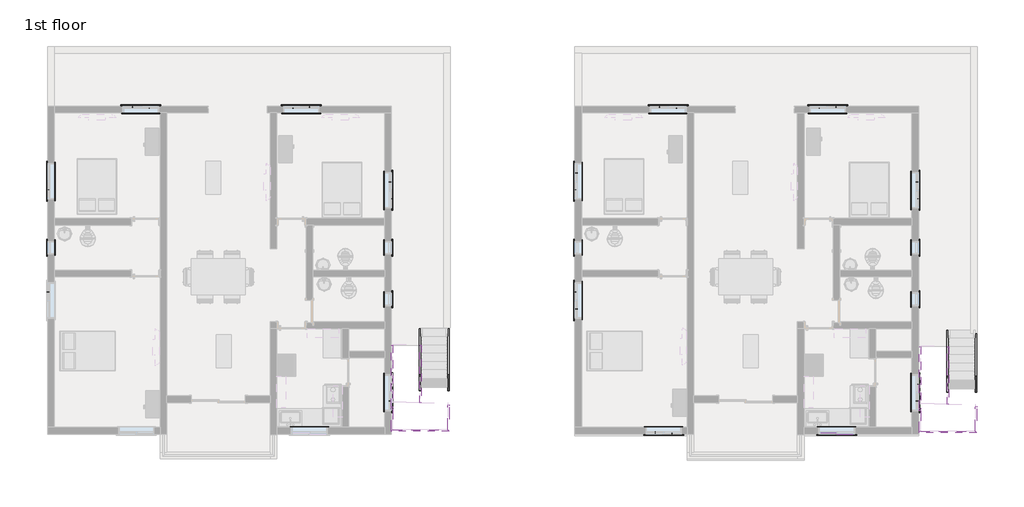
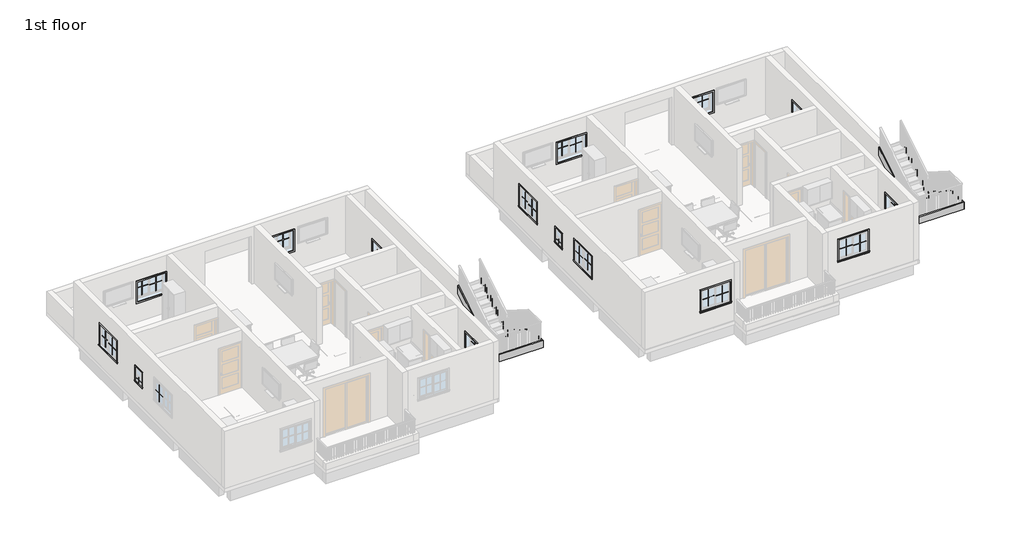
# One storey, part 8 of 8: 72 proxies, 14 members.
"""IFC4 building model written with IfcOpenShell, lengths in millimetres."""

from ifc_helpers import new_model, si_unit, frame, origin, place, context, project, spatial, polyline, outline, extrude, faceted_brep, transform, mapped, element, save
from components import muntin_pattern_2x2_muntin_pattern_2x2_0ac132d2, muntin_pattern_2x2_muntin_pattern_2x2_1fb5fae3, muntin_pattern_2x2_muntin_pattern_2x2_bb7dbb97, trim_window_exterior_flat_with_sill_c4e67c73, trim_window_exterior_flat_with_sill_729ce974, trim_window_exterior_flat_with_sill_e496db69, trim_window_interior_flat_picture_frame_cf1733af, trim_window_interior_flat_picture_frame_5593adf3, trim_window_interior_flat_picture_frame_58837336

model = new_model("IFC4")

# Units and contexts
model_context = context("Model", 3, world=origin())
ifc_project = project(units=[si_unit("LENGTHUNIT", "METRE", prefix="MILLI")], contexts=[model_context])

# Site, building, storey
site = spatial("IfcSite", under=ifc_project)
building = spatial("IfcBuilding", under=site)
storey = spatial("IfcBuildingStorey", under=building, Name="1st floor", Elevation=3810.0)

# Proxies
placement = place(None, origin())
muntin_pattern_2x2_muntin_pattern_2x2_shape = muntin_pattern_2x2_muntin_pattern_2x2_0ac132d2(model_context)
element("IfcBuildingElementProxy", 1, Name="Muntin Pattern_2x2 : Muntin Pattern_2x2", ObjectType="Muntin Pattern_2x2 : Muntin Pattern_2x2", at=placement, inside=storey, context=model_context, shape_type="MappedRepresentation", body=[
    mapped(muntin_pattern_2x2_muntin_pattern_2x2_shape, transform((-12854.1368763, 6465.9185985, 4806.95), x_axis=(1.0, 0.0, 0.0), y_axis=(0.0, 1.0, 0.0), z_axis=(0.0, 0.0, 1.0))),
])
element("IfcBuildingElementProxy", 2, Name="Muntin Pattern_2x2 : Muntin Pattern_2x2", ObjectType="Muntin Pattern_2x2 : Muntin Pattern_2x2", at=placement, inside=storey, context=model_context, shape_type="MappedRepresentation", body=[
    mapped(muntin_pattern_2x2_muntin_pattern_2x2_shape, transform((-13422.4618763, 6510.3685985, 4806.95), x_axis=(1.0, 0.0, 0.0), y_axis=(0.0, 1.0, 0.0), z_axis=(0.0, 0.0, 1.0))),
])
element("IfcBuildingElementProxy", 3, Name="Muntin Pattern_2x2 : Muntin Pattern_2x2", ObjectType="Muntin Pattern_2x2 : Muntin Pattern_2x2", at=placement, inside=storey, context=model_context, shape_type="MappedRepresentation", body=[
    mapped(muntin_pattern_2x2_muntin_pattern_2x2_shape, transform((-16246.6243763, 4251.3560985, 4806.95), x_axis=(0.0, 1.0, 0.0), y_axis=(-1.0, 0.0, 0.0), z_axis=(0.0, 0.0, 1.0))),
])
element("IfcBuildingElementProxy", 4, Name="Muntin Pattern_2x2 : Muntin Pattern_2x2", ObjectType="Muntin Pattern_2x2 : Muntin Pattern_2x2", at=placement, inside=storey, context=model_context, shape_type="MappedRepresentation", body=[
    mapped(muntin_pattern_2x2_muntin_pattern_2x2_shape, transform((-16291.0743763, 3683.0310985, 4806.95), x_axis=(0.0, 1.0, 0.0), y_axis=(-1.0, 0.0, 0.0), z_axis=(0.0, 0.0, 1.0))),
])
element("IfcBuildingElementProxy", 5, Name="Muntin Pattern_2x2 : Muntin Pattern_2x2", ObjectType="Muntin Pattern_2x2 : Muntin Pattern_2x2", at=placement, inside=storey, context=model_context, shape_type="MappedRepresentation", body=[
    mapped(muntin_pattern_2x2_muntin_pattern_2x2_shape, transform((-4695.9743763, -3479.7689015, 4806.95), x_axis=(0.0, -1.0, 0.0), y_axis=(1.0, 0.0, 0.0), z_axis=(0.0, 0.0, 1.0))),
])
element("IfcBuildingElementProxy", 6, Name="Muntin Pattern_2x2 : Muntin Pattern_2x2", ObjectType="Muntin Pattern_2x2 : Muntin Pattern_2x2", at=placement, inside=storey, context=model_context, shape_type="MappedRepresentation", body=[
    mapped(muntin_pattern_2x2_muntin_pattern_2x2_shape, transform((-4651.5243763, -2911.4439015, 4806.95), x_axis=(0.0, -1.0, 0.0), y_axis=(1.0, 0.0, 0.0), z_axis=(0.0, 0.0, 1.0))),
])
element("IfcBuildingElementProxy", 7, Name="Muntin Pattern_2x2 : Muntin Pattern_2x2", ObjectType="Muntin Pattern_2x2 : Muntin Pattern_2x2", at=placement, inside=storey, context=model_context, shape_type="MappedRepresentation", body=[
    mapped(muntin_pattern_2x2_muntin_pattern_2x2_shape, transform((10167.1136273, -4551.3314015, 5035.55), x_axis=(-1.0, 0.0, 0.0), y_axis=(0.0, -1.0, 0.0), z_axis=(0.0, 0.0, 1.0))),
])
element("IfcBuildingElementProxy", 8, Name="Muntin Pattern_2x2 : Muntin Pattern_2x2", ObjectType="Muntin Pattern_2x2 : Muntin Pattern_2x2", at=placement, inside=storey, context=model_context, shape_type="MappedRepresentation", body=[
    mapped(muntin_pattern_2x2_muntin_pattern_2x2_shape, transform((10735.4386273, -4595.7814015, 5035.55), x_axis=(-1.0, 0.0, 0.0), y_axis=(0.0, -1.0, 0.0), z_axis=(0.0, 0.0, 1.0))),
])
element("IfcBuildingElementProxy", 9, Name="Muntin Pattern_2x2 : Muntin Pattern_2x2", ObjectType="Muntin Pattern_2x2 : Muntin Pattern_2x2", at=placement, inside=storey, context=model_context, shape_type="MappedRepresentation", body=[
    mapped(muntin_pattern_2x2_muntin_pattern_2x2_shape, transform((5020.4386273, 6465.9185985, 4806.95), x_axis=(1.0, 0.0, 0.0), y_axis=(0.0, 1.0, 0.0), z_axis=(0.0, 0.0, 1.0))),
])
element("IfcBuildingElementProxy", 10, Name="Muntin Pattern_2x2 : Muntin Pattern_2x2", ObjectType="Muntin Pattern_2x2 : Muntin Pattern_2x2", at=placement, inside=storey, context=model_context, shape_type="MappedRepresentation", body=[
    mapped(muntin_pattern_2x2_muntin_pattern_2x2_shape, transform((4452.1136273, 6510.3685985, 4806.95), x_axis=(1.0, 0.0, 0.0), y_axis=(0.0, 1.0, 0.0), z_axis=(0.0, 0.0, 1.0))),
])
element("IfcBuildingElementProxy", 11, Name="Muntin Pattern_2x2 : Muntin Pattern_2x2", ObjectType="Muntin Pattern_2x2 : Muntin Pattern_2x2", at=placement, inside=storey, context=model_context, shape_type="MappedRepresentation", body=[
    mapped(muntin_pattern_2x2_muntin_pattern_2x2_shape, transform((1627.9511273, 4251.3560985, 4806.95), x_axis=(0.0, 1.0, 0.0), y_axis=(-1.0, 0.0, 0.0), z_axis=(0.0, 0.0, 1.0))),
])
element("IfcBuildingElementProxy", 12, Name="Muntin Pattern_2x2 : Muntin Pattern_2x2", ObjectType="Muntin Pattern_2x2 : Muntin Pattern_2x2", at=placement, inside=storey, context=model_context, shape_type="MappedRepresentation", body=[
    mapped(muntin_pattern_2x2_muntin_pattern_2x2_shape, transform((1583.5011273, 3683.0310985, 4806.95), x_axis=(0.0, 1.0, 0.0), y_axis=(-1.0, 0.0, 0.0), z_axis=(0.0, 0.0, 1.0))),
])
element("IfcBuildingElementProxy", 13, Name="Muntin Pattern_2x2 : Muntin Pattern_2x2", ObjectType="Muntin Pattern_2x2 : Muntin Pattern_2x2", at=placement, inside=storey, context=model_context, shape_type="MappedRepresentation", body=[
    mapped(muntin_pattern_2x2_muntin_pattern_2x2_shape, transform((4299.7136273, -4551.3314015, 4806.95), x_axis=(-1.0, 0.0, 0.0), y_axis=(0.0, -1.0, 0.0), z_axis=(0.0, 0.0, 1.0))),
])
element("IfcBuildingElementProxy", 14, Name="Muntin Pattern_2x2 : Muntin Pattern_2x2", ObjectType="Muntin Pattern_2x2 : Muntin Pattern_2x2", at=placement, inside=storey, context=model_context, shape_type="MappedRepresentation", body=[
    mapped(muntin_pattern_2x2_muntin_pattern_2x2_shape, transform((4868.0386273, -4595.7814015, 4806.95), x_axis=(-1.0, 0.0, 0.0), y_axis=(0.0, -1.0, 0.0), z_axis=(0.0, 0.0, 1.0))),
])
element("IfcBuildingElementProxy", 15, Name="Muntin Pattern_2x2 : Muntin Pattern_2x2", ObjectType="Muntin Pattern_2x2 : Muntin Pattern_2x2", at=placement, inside=storey, context=model_context, shape_type="MappedRepresentation", body=[
    mapped(muntin_pattern_2x2_muntin_pattern_2x2_shape, transform((13178.6011273, -3479.7689015, 4806.95), x_axis=(0.0, -1.0, 0.0), y_axis=(1.0, 0.0, 0.0), z_axis=(0.0, 0.0, 1.0))),
])
element("IfcBuildingElementProxy", 16, Name="Muntin Pattern_2x2 : Muntin Pattern_2x2", ObjectType="Muntin Pattern_2x2 : Muntin Pattern_2x2", at=placement, inside=storey, context=model_context, shape_type="MappedRepresentation", body=[
    mapped(muntin_pattern_2x2_muntin_pattern_2x2_shape, transform((13223.0511273, -2911.4439015, 4806.95), x_axis=(0.0, -1.0, 0.0), y_axis=(1.0, 0.0, 0.0), z_axis=(0.0, 0.0, 1.0))),
])
muntin_pattern_2x2_muntin_pattern_2x2_2_shape = muntin_pattern_2x2_muntin_pattern_2x2_1fb5fae3(model_context)
element("IfcBuildingElementProxy", 17, Name="Muntin Pattern_2x2 : Muntin Pattern_2x2", ObjectType="Muntin Pattern_2x2 : Muntin Pattern_2x2", at=placement, inside=storey, context=model_context, shape_type="MappedRepresentation", body=[
    mapped(muntin_pattern_2x2_muntin_pattern_2x2_2_shape, transform((-4695.9743763, 3946.5560985, 4806.95), x_axis=(0.0, 1.0, 0.0), y_axis=(-1.0, 0.0, 0.0), z_axis=(0.0, 0.0, 1.0))),
])
element("IfcBuildingElementProxy", 18, Name="Muntin Pattern_2x2 : Muntin Pattern_2x2", ObjectType="Muntin Pattern_2x2 : Muntin Pattern_2x2", at=placement, inside=storey, context=model_context, shape_type="MappedRepresentation", body=[
    mapped(muntin_pattern_2x2_muntin_pattern_2x2_2_shape, transform((-4651.5243763, 3378.2310985, 4806.95), x_axis=(0.0, 1.0, 0.0), y_axis=(-1.0, 0.0, 0.0), z_axis=(0.0, 0.0, 1.0))),
])
element("IfcBuildingElementProxy", 19, Name="Muntin Pattern_2x2 : Muntin Pattern_2x2", ObjectType="Muntin Pattern_2x2 : Muntin Pattern_2x2", at=placement, inside=storey, context=model_context, shape_type="MappedRepresentation", body=[
    mapped(muntin_pattern_2x2_muntin_pattern_2x2_2_shape, transform((-7986.8618763, 6465.9185985, 4806.95), x_axis=(-1.0, 0.0, 0.0), y_axis=(0.0, -1.0, 0.0), z_axis=(0.0, 0.0, 1.0))),
])
element("IfcBuildingElementProxy", 20, Name="Muntin Pattern_2x2 : Muntin Pattern_2x2", ObjectType="Muntin Pattern_2x2 : Muntin Pattern_2x2", at=placement, inside=storey, context=model_context, shape_type="MappedRepresentation", body=[
    mapped(muntin_pattern_2x2_muntin_pattern_2x2_2_shape, transform((-7418.5368763, 6510.3685985, 4806.95), x_axis=(-1.0, 0.0, 0.0), y_axis=(0.0, -1.0, 0.0), z_axis=(0.0, 0.0, 1.0))),
])
element("IfcBuildingElementProxy", 21, Name="Muntin Pattern_2x2 : Muntin Pattern_2x2", ObjectType="Muntin Pattern_2x2 : Muntin Pattern_2x2", at=placement, inside=storey, context=model_context, shape_type="MappedRepresentation", body=[
    mapped(muntin_pattern_2x2_muntin_pattern_2x2_2_shape, transform((-16291.0743763, 212.7560985, 4806.95), x_axis=(0.0, -1.0, 0.0), y_axis=(1.0, 0.0, 0.0), z_axis=(0.0, 0.0, 1.0))),
])
element("IfcBuildingElementProxy", 22, Name="Muntin Pattern_2x2 : Muntin Pattern_2x2", ObjectType="Muntin Pattern_2x2 : Muntin Pattern_2x2", at=placement, inside=storey, context=model_context, shape_type="MappedRepresentation", body=[
    mapped(muntin_pattern_2x2_muntin_pattern_2x2_2_shape, transform((13178.6011273, 3946.5560985, 4806.95), x_axis=(0.0, 1.0, 0.0), y_axis=(-1.0, 0.0, 0.0), z_axis=(0.0, 0.0, 1.0))),
])
element("IfcBuildingElementProxy", 23, Name="Muntin Pattern_2x2 : Muntin Pattern_2x2", ObjectType="Muntin Pattern_2x2 : Muntin Pattern_2x2", at=placement, inside=storey, context=model_context, shape_type="MappedRepresentation", body=[
    mapped(muntin_pattern_2x2_muntin_pattern_2x2_2_shape, transform((13223.0511273, 3378.2310985, 4806.95), x_axis=(0.0, 1.0, 0.0), y_axis=(-1.0, 0.0, 0.0), z_axis=(0.0, 0.0, 1.0))),
])
element("IfcBuildingElementProxy", 24, Name="Muntin Pattern_2x2 : Muntin Pattern_2x2", ObjectType="Muntin Pattern_2x2 : Muntin Pattern_2x2", at=placement, inside=storey, context=model_context, shape_type="MappedRepresentation", body=[
    mapped(muntin_pattern_2x2_muntin_pattern_2x2_2_shape, transform((9862.3136273, 6465.9185985, 4806.95), x_axis=(-1.0, 0.0, 0.0), y_axis=(0.0, -1.0, 0.0), z_axis=(0.0, 0.0, 1.0))),
])
element("IfcBuildingElementProxy", 25, Name="Muntin Pattern_2x2 : Muntin Pattern_2x2", ObjectType="Muntin Pattern_2x2 : Muntin Pattern_2x2", at=placement, inside=storey, context=model_context, shape_type="MappedRepresentation", body=[
    mapped(muntin_pattern_2x2_muntin_pattern_2x2_2_shape, transform((10430.6386273, 6510.3685985, 4806.95), x_axis=(-1.0, 0.0, 0.0), y_axis=(0.0, -1.0, 0.0), z_axis=(0.0, 0.0, 1.0))),
])
element("IfcBuildingElementProxy", 26, Name="Muntin Pattern_2x2 : Muntin Pattern_2x2", ObjectType="Muntin Pattern_2x2 : Muntin Pattern_2x2", at=placement, inside=storey, context=model_context, shape_type="MappedRepresentation", body=[
    mapped(muntin_pattern_2x2_muntin_pattern_2x2_2_shape, transform((1627.9511273, -355.5689015, 4806.95), x_axis=(0.0, -1.0, 0.0), y_axis=(1.0, 0.0, 0.0), z_axis=(0.0, 0.0, 1.0))),
])
element("IfcBuildingElementProxy", 27, Name="Muntin Pattern_2x2 : Muntin Pattern_2x2", ObjectType="Muntin Pattern_2x2 : Muntin Pattern_2x2", at=placement, inside=storey, context=model_context, shape_type="MappedRepresentation", body=[
    mapped(muntin_pattern_2x2_muntin_pattern_2x2_2_shape, transform((1583.5011273, 212.7560985, 4806.95), x_axis=(0.0, -1.0, 0.0), y_axis=(1.0, 0.0, 0.0), z_axis=(0.0, 0.0, 1.0))),
])
muntin_pattern_2x2_muntin_pattern_2x2_3_shape = muntin_pattern_2x2_muntin_pattern_2x2_bb7dbb97(model_context)
element("IfcBuildingElementProxy", 28, Name="Muntin Pattern_2x2 : Muntin Pattern_2x2", ObjectType="Muntin Pattern_2x2 : Muntin Pattern_2x2", at=placement, inside=storey, context=model_context, shape_type="MappedRepresentation", body=[
    mapped(muntin_pattern_2x2_muntin_pattern_2x2_3_shape, transform((-4651.5243763, -33.3064015, 4762.5), x_axis=(0.0, 1.0, 0.0), y_axis=(-1.0, 0.0, 0.0), z_axis=(0.0, 0.0, 1.0))),
])
element("IfcBuildingElementProxy", 29, Name="Muntin Pattern_2x2 : Muntin Pattern_2x2", ObjectType="Muntin Pattern_2x2 : Muntin Pattern_2x2", at=placement, inside=storey, context=model_context, shape_type="MappedRepresentation", body=[
    mapped(muntin_pattern_2x2_muntin_pattern_2x2_3_shape, transform((-4651.5243763, 1719.2935985, 4762.5), x_axis=(0.0, 1.0, 0.0), y_axis=(-1.0, 0.0, 0.0), z_axis=(0.0, 0.0, 1.0))),
])
element("IfcBuildingElementProxy", 30, Name="Muntin Pattern_2x2 : Muntin Pattern_2x2", ObjectType="Muntin Pattern_2x2 : Muntin Pattern_2x2", at=placement, inside=storey, context=model_context, shape_type="MappedRepresentation", body=[
    mapped(muntin_pattern_2x2_muntin_pattern_2x2_3_shape, transform((-16291.0743763, 1719.2935985, 4762.5), x_axis=(0.0, -1.0, 0.0), y_axis=(1.0, 0.0, 0.0), z_axis=(0.0, 0.0, 1.0))),
])
element("IfcBuildingElementProxy", 31, Name="Muntin Pattern_2x2 : Muntin Pattern_2x2", ObjectType="Muntin Pattern_2x2 : Muntin Pattern_2x2", at=placement, inside=storey, context=model_context, shape_type="MappedRepresentation", body=[
    mapped(muntin_pattern_2x2_muntin_pattern_2x2_3_shape, transform((13223.0511273, -33.3064015, 4762.5), x_axis=(0.0, 1.0, 0.0), y_axis=(-1.0, 0.0, 0.0), z_axis=(0.0, 0.0, 1.0))),
])
element("IfcBuildingElementProxy", 32, Name="Muntin Pattern_2x2 : Muntin Pattern_2x2", ObjectType="Muntin Pattern_2x2 : Muntin Pattern_2x2", at=placement, inside=storey, context=model_context, shape_type="MappedRepresentation", body=[
    mapped(muntin_pattern_2x2_muntin_pattern_2x2_3_shape, transform((13223.0511273, 1719.2935985, 4762.5), x_axis=(0.0, 1.0, 0.0), y_axis=(-1.0, 0.0, 0.0), z_axis=(0.0, 0.0, 1.0))),
])
element("IfcBuildingElementProxy", 33, Name="Muntin Pattern_2x2 : Muntin Pattern_2x2", ObjectType="Muntin Pattern_2x2 : Muntin Pattern_2x2", at=placement, inside=storey, context=model_context, shape_type="MappedRepresentation", body=[
    mapped(muntin_pattern_2x2_muntin_pattern_2x2_3_shape, transform((1583.5011273, 1719.2935985, 4762.5), x_axis=(0.0, -1.0, 0.0), y_axis=(1.0, 0.0, 0.0), z_axis=(0.0, 0.0, 1.0))),
])
trim_window_exterior_flat_with_sill_shape = trim_window_exterior_flat_with_sill_c4e67c73(model_context)
element("IfcBuildingElementProxy", 34, Name="Trim-Window-Exterior-Flat : with Sill", ObjectType="Trim-Window-Exterior-Flat : with Sill", at=placement, inside=storey, context=model_context, shape_type="MappedRepresentation", body=[
    mapped(trim_window_exterior_flat_with_sill_shape, transform((-13138.2993763, 6519.8935985, 5638.8), x_axis=(-1.0, 0.0, 0.0), y_axis=(0.0, 0.0, 1.0), z_axis=(0.0, 1.0, 0.0))),
])
element("IfcBuildingElementProxy", 35, Name="Trim-Window-Exterior-Flat : with Sill", ObjectType="Trim-Window-Exterior-Flat : with Sill", at=placement, inside=storey, context=model_context, shape_type="MappedRepresentation", body=[
    mapped(trim_window_exterior_flat_with_sill_shape, transform((-16300.5993763, 3967.1935985, 5638.8), x_axis=(0.0, -1.0, 0.0), y_axis=(0.0, 0.0, 1.0), z_axis=(-1.0, 0.0, 0.0))),
])
element("IfcBuildingElementProxy", 36, Name="Trim-Window-Exterior-Flat : with Sill", ObjectType="Trim-Window-Exterior-Flat : with Sill", at=placement, inside=storey, context=model_context, shape_type="MappedRepresentation", body=[
    mapped(trim_window_exterior_flat_with_sill_shape, transform((-4641.9993763, -3195.6064015, 5638.8), x_axis=(0.0, 1.0, 0.0), y_axis=(0.0, 0.0, 1.0), z_axis=(1.0, 0.0, 0.0))),
])
element("IfcBuildingElementProxy", 37, Name="Trim-Window-Exterior-Flat : with Sill", ObjectType="Trim-Window-Exterior-Flat : with Sill", at=placement, inside=storey, context=model_context, shape_type="MappedRepresentation", body=[
    mapped(trim_window_exterior_flat_with_sill_shape, transform((10451.2761273, -4605.3064015, 5867.4), x_axis=(1.0, 0.0, 0.0), y_axis=(0.0, 0.0, 1.0), z_axis=(0.0, -1.0, 0.0))),
])
element("IfcBuildingElementProxy", 38, Name="Trim-Window-Exterior-Flat : with Sill", ObjectType="Trim-Window-Exterior-Flat : with Sill", at=placement, inside=storey, context=model_context, shape_type="MappedRepresentation", body=[
    mapped(trim_window_exterior_flat_with_sill_shape, transform((4736.2761273, 6519.8935985, 5638.8), x_axis=(-1.0, 0.0, 0.0), y_axis=(0.0, 0.0, 1.0), z_axis=(0.0, 1.0, 0.0))),
])
element("IfcBuildingElementProxy", 39, Name="Trim-Window-Exterior-Flat : with Sill", ObjectType="Trim-Window-Exterior-Flat : with Sill", at=placement, inside=storey, context=model_context, shape_type="MappedRepresentation", body=[
    mapped(trim_window_exterior_flat_with_sill_shape, transform((1573.9761273, 3967.1935985, 5638.8), x_axis=(0.0, -1.0, 0.0), y_axis=(0.0, 0.0, 1.0), z_axis=(-1.0, 0.0, 0.0))),
])
element("IfcBuildingElementProxy", 40, Name="Trim-Window-Exterior-Flat : with Sill", ObjectType="Trim-Window-Exterior-Flat : with Sill", at=placement, inside=storey, context=model_context, shape_type="MappedRepresentation", body=[
    mapped(trim_window_exterior_flat_with_sill_shape, transform((4583.8761273, -4605.3064015, 5638.8), x_axis=(1.0, 0.0, 0.0), y_axis=(0.0, 0.0, 1.0), z_axis=(0.0, -1.0, 0.0))),
])
element("IfcBuildingElementProxy", 41, Name="Trim-Window-Exterior-Flat : with Sill", ObjectType="Trim-Window-Exterior-Flat : with Sill", at=placement, inside=storey, context=model_context, shape_type="MappedRepresentation", body=[
    mapped(trim_window_exterior_flat_with_sill_shape, transform((13232.5761273, -3195.6064015, 5638.8), x_axis=(0.0, 1.0, 0.0), y_axis=(0.0, 0.0, 1.0), z_axis=(1.0, 0.0, 0.0))),
])
trim_window_exterior_flat_with_sill_2_shape = trim_window_exterior_flat_with_sill_729ce974(model_context)
element("IfcBuildingElementProxy", 42, Name="Trim-Window-Exterior-Flat : with Sill", ObjectType="Trim-Window-Exterior-Flat : with Sill", at=placement, inside=storey, context=model_context, shape_type="MappedRepresentation", body=[
    mapped(trim_window_exterior_flat_with_sill_2_shape, transform((-4641.9993763, 3662.3935985, 5638.8), x_axis=(0.0, -1.0, 0.0), y_axis=(0.0, 0.0, -1.0), z_axis=(1.0, 0.0, 0.0))),
])
element("IfcBuildingElementProxy", 43, Name="Trim-Window-Exterior-Flat : with Sill", ObjectType="Trim-Window-Exterior-Flat : with Sill", at=placement, inside=storey, context=model_context, shape_type="MappedRepresentation", body=[
    mapped(trim_window_exterior_flat_with_sill_2_shape, transform((-7702.6993763, 6519.8935985, 5638.8), x_axis=(1.0, 0.0, 0.0), y_axis=(0.0, 0.0, -1.0), z_axis=(0.0, 1.0, 0.0))),
])
element("IfcBuildingElementProxy", 44, Name="Trim-Window-Exterior-Flat : with Sill", ObjectType="Trim-Window-Exterior-Flat : with Sill", at=placement, inside=storey, context=model_context, shape_type="MappedRepresentation", body=[
    mapped(trim_window_exterior_flat_with_sill_2_shape, transform((13232.5761273, 3662.3935985, 5638.8), x_axis=(0.0, -1.0, 0.0), y_axis=(0.0, 0.0, -1.0), z_axis=(1.0, 0.0, 0.0))),
])
element("IfcBuildingElementProxy", 45, Name="Trim-Window-Exterior-Flat : with Sill", ObjectType="Trim-Window-Exterior-Flat : with Sill", at=placement, inside=storey, context=model_context, shape_type="MappedRepresentation", body=[
    mapped(trim_window_exterior_flat_with_sill_2_shape, transform((10146.4761273, 6519.8935985, 5638.8), x_axis=(1.0, 0.0, 0.0), y_axis=(0.0, 0.0, -1.0), z_axis=(0.0, 1.0, 0.0))),
])
element("IfcBuildingElementProxy", 46, Name="Trim-Window-Exterior-Flat : with Sill", ObjectType="Trim-Window-Exterior-Flat : with Sill", at=placement, inside=storey, context=model_context, shape_type="MappedRepresentation", body=[
    mapped(trim_window_exterior_flat_with_sill_2_shape, transform((1573.9761273, -71.4064015, 5638.8), x_axis=(0.0, 1.0, 0.0), y_axis=(0.0, 0.0, -1.0), z_axis=(-1.0, 0.0, 0.0))),
])
trim_window_exterior_flat_with_sill_3_shape = trim_window_exterior_flat_with_sill_e496db69(model_context)
element("IfcBuildingElementProxy", 47, Name="Trim-Window-Exterior-Flat : with Sill", ObjectType="Trim-Window-Exterior-Flat : with Sill", at=placement, inside=storey, context=model_context, shape_type="MappedRepresentation", body=[
    mapped(trim_window_exterior_flat_with_sill_3_shape, transform((-4641.9993763, -33.3064015, 5334.0), x_axis=(0.0, 1.0, 0.0), y_axis=(0.0, 0.0, 1.0), z_axis=(1.0, 0.0, 0.0))),
])
element("IfcBuildingElementProxy", 48, Name="Trim-Window-Exterior-Flat : with Sill", ObjectType="Trim-Window-Exterior-Flat : with Sill", at=placement, inside=storey, context=model_context, shape_type="MappedRepresentation", body=[
    mapped(trim_window_exterior_flat_with_sill_3_shape, transform((-4641.9993763, 1719.2935985, 5334.0), x_axis=(0.0, 1.0, 0.0), y_axis=(0.0, 0.0, 1.0), z_axis=(1.0, 0.0, 0.0))),
])
element("IfcBuildingElementProxy", 49, Name="Trim-Window-Exterior-Flat : with Sill", ObjectType="Trim-Window-Exterior-Flat : with Sill", at=placement, inside=storey, context=model_context, shape_type="MappedRepresentation", body=[
    mapped(trim_window_exterior_flat_with_sill_3_shape, transform((-16300.5993763, 1719.2935985, 5334.0), x_axis=(0.0, -1.0, 0.0), y_axis=(0.0, 0.0, 1.0), z_axis=(-1.0, 0.0, 0.0))),
])
element("IfcBuildingElementProxy", 50, Name="Trim-Window-Exterior-Flat : with Sill", ObjectType="Trim-Window-Exterior-Flat : with Sill", at=placement, inside=storey, context=model_context, shape_type="MappedRepresentation", body=[
    mapped(trim_window_exterior_flat_with_sill_3_shape, transform((13232.5761273, -33.3064015, 5334.0), x_axis=(0.0, 1.0, 0.0), y_axis=(0.0, 0.0, 1.0), z_axis=(1.0, 0.0, 0.0))),
])
element("IfcBuildingElementProxy", 51, Name="Trim-Window-Exterior-Flat : with Sill", ObjectType="Trim-Window-Exterior-Flat : with Sill", at=placement, inside=storey, context=model_context, shape_type="MappedRepresentation", body=[
    mapped(trim_window_exterior_flat_with_sill_3_shape, transform((13232.5761273, 1719.2935985, 5334.0), x_axis=(0.0, 1.0, 0.0), y_axis=(0.0, 0.0, 1.0), z_axis=(1.0, 0.0, 0.0))),
])
element("IfcBuildingElementProxy", 52, Name="Trim-Window-Exterior-Flat : with Sill", ObjectType="Trim-Window-Exterior-Flat : with Sill", at=placement, inside=storey, context=model_context, shape_type="MappedRepresentation", body=[
    mapped(trim_window_exterior_flat_with_sill_3_shape, transform((1573.9761273, 1719.2935985, 5334.0), x_axis=(0.0, -1.0, 0.0), y_axis=(0.0, 0.0, 1.0), z_axis=(-1.0, 0.0, 0.0))),
])
trim_window_interior_flat_picture_frame_shape = trim_window_interior_flat_picture_frame_cf1733af(model_context)
element("IfcBuildingElementProxy", 53, Name="Trim-Window-Interior-Flat : Picture Frame", ObjectType="Trim-Window-Interior-Flat : Picture Frame", at=placement, inside=storey, context=model_context, shape_type="MappedRepresentation", body=[
    mapped(trim_window_interior_flat_picture_frame_shape, transform((-7423.2993763, -4376.7064015, 5867.4), x_axis=(-1.0, 0.0, 0.0), y_axis=(0.0, 0.0, 1.0), z_axis=(0.0, 1.0, 0.0))),
])
element("IfcBuildingElementProxy", 54, Name="Trim-Window-Interior-Flat : Picture Frame", ObjectType="Trim-Window-Interior-Flat : Picture Frame", at=placement, inside=storey, context=model_context, shape_type="MappedRepresentation", body=[
    mapped(trim_window_interior_flat_picture_frame_shape, transform((-13138.2993763, 6291.2935985, 5638.8), x_axis=(1.0, 0.0, 0.0), y_axis=(0.0, 0.0, 1.0), z_axis=(0.0, -1.0, 0.0))),
])
element("IfcBuildingElementProxy", 55, Name="Trim-Window-Interior-Flat : Picture Frame", ObjectType="Trim-Window-Interior-Flat : Picture Frame", at=placement, inside=storey, context=model_context, shape_type="MappedRepresentation", body=[
    mapped(trim_window_interior_flat_picture_frame_shape, transform((-16071.9993763, 3967.1935985, 5638.8), x_axis=(0.0, 1.0, 0.0), y_axis=(0.0, 0.0, 1.0), z_axis=(1.0, 0.0, 0.0))),
])
element("IfcBuildingElementProxy", 56, Name="Trim-Window-Interior-Flat : Picture Frame", ObjectType="Trim-Window-Interior-Flat : Picture Frame", at=placement, inside=storey, context=model_context, shape_type="MappedRepresentation", body=[
    mapped(trim_window_interior_flat_picture_frame_shape, transform((-4870.5993763, -3195.6064015, 5638.8), x_axis=(0.0, -1.0, 0.0), y_axis=(0.0, 0.0, 1.0), z_axis=(-1.0, 0.0, 0.0))),
])
element("IfcBuildingElementProxy", 57, Name="Trim-Window-Interior-Flat : Picture Frame", ObjectType="Trim-Window-Interior-Flat : Picture Frame", at=placement, inside=storey, context=model_context, shape_type="MappedRepresentation", body=[
    mapped(trim_window_interior_flat_picture_frame_shape, transform((10451.2761273, -4376.7064015, 5867.4), x_axis=(-1.0, 0.0, 0.0), y_axis=(0.0, 0.0, 1.0), z_axis=(0.0, 1.0, 0.0))),
])
element("IfcBuildingElementProxy", 58, Name="Trim-Window-Interior-Flat : Picture Frame", ObjectType="Trim-Window-Interior-Flat : Picture Frame", at=placement, inside=storey, context=model_context, shape_type="MappedRepresentation", body=[
    mapped(trim_window_interior_flat_picture_frame_shape, transform((4736.2761273, 6291.2935985, 5638.8), x_axis=(1.0, 0.0, 0.0), y_axis=(0.0, 0.0, 1.0), z_axis=(0.0, -1.0, 0.0))),
])
element("IfcBuildingElementProxy", 59, Name="Trim-Window-Interior-Flat : Picture Frame", ObjectType="Trim-Window-Interior-Flat : Picture Frame", at=placement, inside=storey, context=model_context, shape_type="MappedRepresentation", body=[
    mapped(trim_window_interior_flat_picture_frame_shape, transform((1802.5761273, 3967.1935985, 5638.8), x_axis=(0.0, 1.0, 0.0), y_axis=(0.0, 0.0, 1.0), z_axis=(1.0, 0.0, 0.0))),
])
element("IfcBuildingElementProxy", 60, Name="Trim-Window-Interior-Flat : Picture Frame", ObjectType="Trim-Window-Interior-Flat : Picture Frame", at=placement, inside=storey, context=model_context, shape_type="MappedRepresentation", body=[
    mapped(trim_window_interior_flat_picture_frame_shape, transform((4583.8761273, -4376.7064015, 5638.8), x_axis=(-1.0, 0.0, 0.0), y_axis=(0.0, 0.0, 1.0), z_axis=(0.0, 1.0, 0.0))),
])
element("IfcBuildingElementProxy", 61, Name="Trim-Window-Interior-Flat : Picture Frame", ObjectType="Trim-Window-Interior-Flat : Picture Frame", at=placement, inside=storey, context=model_context, shape_type="MappedRepresentation", body=[
    mapped(trim_window_interior_flat_picture_frame_shape, transform((13003.9761273, -3195.6064015, 5638.8), x_axis=(0.0, -1.0, 0.0), y_axis=(0.0, 0.0, 1.0), z_axis=(-1.0, 0.0, 0.0))),
])
trim_window_interior_flat_picture_frame_2_shape = trim_window_interior_flat_picture_frame_5593adf3(model_context)
element("IfcBuildingElementProxy", 62, Name="Trim-Window-Interior-Flat : Picture Frame", ObjectType="Trim-Window-Interior-Flat : Picture Frame", at=placement, inside=storey, context=model_context, shape_type="MappedRepresentation", body=[
    mapped(trim_window_interior_flat_picture_frame_2_shape, transform((-4870.5993763, 3662.3935985, 5638.8), x_axis=(0.0, 1.0, 0.0), y_axis=(0.0, 0.0, -1.0), z_axis=(-1.0, 0.0, 0.0))),
])
element("IfcBuildingElementProxy", 63, Name="Trim-Window-Interior-Flat : Picture Frame", ObjectType="Trim-Window-Interior-Flat : Picture Frame", at=placement, inside=storey, context=model_context, shape_type="MappedRepresentation", body=[
    mapped(trim_window_interior_flat_picture_frame_2_shape, transform((-7702.6993763, 6291.2935985, 5638.8), x_axis=(-1.0, 0.0, 0.0), y_axis=(0.0, 0.0, -1.0), z_axis=(0.0, -1.0, 0.0))),
])
element("IfcBuildingElementProxy", 64, Name="Trim-Window-Interior-Flat : Picture Frame", ObjectType="Trim-Window-Interior-Flat : Picture Frame", at=placement, inside=storey, context=model_context, shape_type="MappedRepresentation", body=[
    mapped(trim_window_interior_flat_picture_frame_2_shape, transform((13003.9761273, 3662.3935985, 5638.8), x_axis=(0.0, 1.0, 0.0), y_axis=(0.0, 0.0, -1.0), z_axis=(-1.0, 0.0, 0.0))),
])
element("IfcBuildingElementProxy", 65, Name="Trim-Window-Interior-Flat : Picture Frame", ObjectType="Trim-Window-Interior-Flat : Picture Frame", at=placement, inside=storey, context=model_context, shape_type="MappedRepresentation", body=[
    mapped(trim_window_interior_flat_picture_frame_2_shape, transform((10146.4761273, 6291.2935985, 5638.8), x_axis=(-1.0, 0.0, 0.0), y_axis=(0.0, 0.0, -1.0), z_axis=(0.0, -1.0, 0.0))),
])
element("IfcBuildingElementProxy", 66, Name="Trim-Window-Interior-Flat : Picture Frame", ObjectType="Trim-Window-Interior-Flat : Picture Frame", at=placement, inside=storey, context=model_context, shape_type="MappedRepresentation", body=[
    mapped(trim_window_interior_flat_picture_frame_2_shape, transform((1802.5761273, -71.4064015, 5638.8), x_axis=(0.0, -1.0, 0.0), y_axis=(0.0, 0.0, -1.0), z_axis=(1.0, 0.0, 0.0))),
])
trim_window_interior_flat_picture_frame_3_shape = trim_window_interior_flat_picture_frame_58837336(model_context)
element("IfcBuildingElementProxy", 67, Name="Trim-Window-Interior-Flat : Picture Frame", ObjectType="Trim-Window-Interior-Flat : Picture Frame", at=placement, inside=storey, context=model_context, shape_type="MappedRepresentation", body=[
    mapped(trim_window_interior_flat_picture_frame_3_shape, transform((-4870.5993763, -33.3064015, 5334.0), x_axis=(0.0, -1.0, 0.0), y_axis=(0.0, 0.0, 1.0), z_axis=(-1.0, 0.0, 0.0))),
])
element("IfcBuildingElementProxy", 68, Name="Trim-Window-Interior-Flat : Picture Frame", ObjectType="Trim-Window-Interior-Flat : Picture Frame", at=placement, inside=storey, context=model_context, shape_type="MappedRepresentation", body=[
    mapped(trim_window_interior_flat_picture_frame_3_shape, transform((-4870.5993763, 1719.2935985, 5334.0), x_axis=(0.0, -1.0, 0.0), y_axis=(0.0, 0.0, 1.0), z_axis=(-1.0, 0.0, 0.0))),
])
element("IfcBuildingElementProxy", 69, Name="Trim-Window-Interior-Flat : Picture Frame", ObjectType="Trim-Window-Interior-Flat : Picture Frame", at=placement, inside=storey, context=model_context, shape_type="MappedRepresentation", body=[
    mapped(trim_window_interior_flat_picture_frame_3_shape, transform((-16071.9993763, 1719.2935985, 5334.0), x_axis=(0.0, 1.0, 0.0), y_axis=(0.0, 0.0, 1.0), z_axis=(1.0, 0.0, 0.0))),
])
element("IfcBuildingElementProxy", 70, Name="Trim-Window-Interior-Flat : Picture Frame", ObjectType="Trim-Window-Interior-Flat : Picture Frame", at=placement, inside=storey, context=model_context, shape_type="MappedRepresentation", body=[
    mapped(trim_window_interior_flat_picture_frame_3_shape, transform((13003.9761273, -33.3064015, 5334.0), x_axis=(0.0, -1.0, 0.0), y_axis=(0.0, 0.0, 1.0), z_axis=(-1.0, 0.0, 0.0))),
])
element("IfcBuildingElementProxy", 71, Name="Trim-Window-Interior-Flat : Picture Frame", ObjectType="Trim-Window-Interior-Flat : Picture Frame", at=placement, inside=storey, context=model_context, shape_type="MappedRepresentation", body=[
    mapped(trim_window_interior_flat_picture_frame_3_shape, transform((13003.9761273, 1719.2935985, 5334.0), x_axis=(0.0, -1.0, 0.0), y_axis=(0.0, 0.0, 1.0), z_axis=(-1.0, 0.0, 0.0))),
])
element("IfcBuildingElementProxy", 72, Name="Trim-Window-Interior-Flat : Picture Frame", ObjectType="Trim-Window-Interior-Flat : Picture Frame", at=placement, inside=storey, context=model_context, shape_type="MappedRepresentation", body=[
    mapped(trim_window_interior_flat_picture_frame_3_shape, transform((1802.5761273, 1719.2935985, 5334.0), x_axis=(0.0, 1.0, 0.0), y_axis=(0.0, 0.0, 1.0), z_axis=(1.0, 0.0, 0.0))),
])

# Members
element("IfcMember", 73, ObjectType="Stringer - 2\" Width", at=placement, inside=storey, context=model_context, shape_type="SweptSolid", body=[
    extrude(outline(polyline([(-1023.9064015, 4025.0106437), (-1023.9064015, 3810.0), (-1253.7619309, 3810.0), (-3688.5333594, 5359.4), (-3599.77539, 5664.2), (-1023.9064015, 4025.0106437)])), frame((-2736.9993763, 0.0, 0.0), z_axis=(1.0, 0.0, 0.0), x_axis=(0.0, 1.0, 0.0)), (0.0, 0.0, 1.0), 50.8),
])
element("IfcMember", 74, ObjectType="Stringer - 2\" Width", at=placement, inside=storey, context=model_context, shape_type="SweptSolid", body=[
    extrude(outline(polyline([(-1023.9064015, 4025.0106437), (-1023.9064015, 3810.0), (-1253.7619309, 3810.0), (-3487.7064015, 5231.6010268), (-3487.7064015, 5592.883371), (-1023.9064015, 4025.0106437)])), frame((-3702.1993763, 0.0, 0.0), z_axis=(1.0, 0.0, 0.0), x_axis=(0.0, 1.0, 0.0)), (0.0, 0.0, 1.0), 50.8),
])
element("IfcMember", 75, ObjectType="Stringer - 2\" Width", at=placement, inside=storey, context=model_context, shape_type="SweptSolid", body=[
    extrude(outline(polyline([(-3667.8794436, 5359.4), (-3756.637413, 5664.2), (-1582.7064015, 7047.6106437), (-1582.7064015, 6686.3282995), (-3667.8794436, 5359.4)])), frame((-4641.9993763, 0.0, 0.0), z_axis=(1.0, 0.0, 0.0), x_axis=(0.0, 1.0, 0.0)), (0.0, 0.0, 1.0), 50.8),
])
element("IfcMember", 76, ObjectType="Stringer - 2\" Width", at=placement, inside=storey, context=model_context, shape_type="SweptSolid", body=[
    extrude(outline(polyline([(-3538.5064015, 5441.7282995), (-3538.5064015, 5803.0106437), (-1582.7064015, 7047.6106437), (-1582.7064015, 6686.3282995), (-3538.5064015, 5441.7282995)])), frame((-3676.7993763, 0.0, 0.0), z_axis=(1.0, 0.0, 0.0), x_axis=(0.0, 1.0, 0.0)), (0.0, 0.0, 1.0), 50.8),
])
element("IfcMember", 77, ObjectType="Stringer - 2\" Width", at=placement, inside=storey, context=model_context, shape_type="Brep", body=[
    faceted_brep([(-4591.1993763, -3756.637413, 5664.2), (-4641.9993763, -3756.637413, 5664.2), (-4641.9993763, -4503.7064015, 5664.2), (-4591.1993763, -4452.9064015, 5664.2), (-4591.1993763, -3667.8794436, 5359.4), (-4591.1993763, -4452.9064015, 5359.4), (-4641.9993763, -3667.8794436, 5359.4), (-4641.9993763, -4503.7064015, 5359.4)], [[[0, 1, 2, 3]], [[4, 0, 3, 5]], [[6, 4, 5, 7]], [[1, 6, 7, 2]], [[1, 0, 4, 6]], [[2, 7, 5, 3]]]),
])
element("IfcMember", 78, ObjectType="Stringer - 2\" Width", at=placement, inside=storey, context=model_context, shape_type="SweptSolid", body=[
    extrude(outline(polyline([(-4641.9993763, -4503.7064015), (-4591.1993763, -4452.9064015), (-2736.9993763, -4452.9064015), (-2686.1993763, -4503.7064015), (-4641.9993763, -4503.7064015)])), frame((0.0, 0.0, 5359.4), z_axis=(0.0, 0.0, 1.0), x_axis=(1.0, 0.0, 0.0)), (0.0, 0.0, 1.0), 304.8),
])
element("IfcMember", 79, ObjectType="Stringer - 2\" Width", at=placement, inside=storey, context=model_context, shape_type="Brep", body=[
    faceted_brep([(-2736.9993763, -4452.9064015, 5664.2), (-2686.1993763, -4503.7064015, 5664.2), (-2686.1993763, -3599.77539, 5664.2), (-2736.9993763, -3599.77539, 5664.2), (-2736.9993763, -4452.9064015, 5359.4), (-2736.9993763, -3688.5333594, 5359.4), (-2686.1993763, -4503.7064015, 5359.4), (-2686.1993763, -3688.5333594, 5359.4)], [[[0, 1, 2, 3]], [[4, 0, 3, 5]], [[6, 4, 5, 7]], [[1, 6, 7, 2]], [[1, 0, 4, 6]], [[2, 7, 5, 3]]]),
])
element("IfcMember", 80, ObjectType="Stringer - 2\" Width", at=placement, inside=storey, context=model_context, shape_type="SweptSolid", body=[
    extrude(outline(polyline([(-1074.7064015, 4025.0106437), (-1074.7064015, 3810.0), (-1304.5619309, 3810.0), (-3739.3333594, 5359.4), (-3650.57539, 5664.2), (-1074.7064015, 4025.0106437)])), frame((15150.9506237, 0.0, 0.0), z_axis=(1.0, 0.0, 0.0), x_axis=(0.0, 1.0, 0.0)), (0.0, 0.0, 1.0), 50.8),
])
element("IfcMember", 81, ObjectType="Stringer - 2\" Width", at=placement, inside=storey, context=model_context, shape_type="SweptSolid", body=[
    extrude(outline(polyline([(-1074.7064015, 4025.0106437), (-1074.7064015, 3810.0), (-1304.5619309, 3810.0), (-3538.5064015, 5231.6010268), (-3538.5064015, 5592.883371), (-1074.7064015, 4025.0106437)])), frame((14185.7506237, 0.0, 0.0), z_axis=(1.0, 0.0, 0.0), x_axis=(0.0, 1.0, 0.0)), (0.0, 0.0, 1.0), 50.8),
])
element("IfcMember", 82, ObjectType="Stringer - 2\" Width", at=placement, inside=storey, context=model_context, shape_type="SweptSolid", body=[
    extrude(outline(polyline([(-3718.6794436, 5359.4), (-3807.437413, 5664.2), (-1633.5064015, 7047.6106437), (-1633.5064015, 6686.3282995), (-3718.6794436, 5359.4)])), frame((13245.9506237, 0.0, 0.0), z_axis=(1.0, 0.0, 0.0), x_axis=(0.0, 1.0, 0.0)), (0.0, 0.0, 1.0), 50.8),
])
element("IfcMember", 83, ObjectType="Stringer - 2\" Width", at=placement, inside=storey, context=model_context, shape_type="SweptSolid", body=[
    extrude(outline(polyline([(-3589.3064015, 5441.7282995), (-3589.3064015, 5803.0106437), (-1633.5064015, 7047.6106437), (-1633.5064015, 6686.3282995), (-3589.3064015, 5441.7282995)])), frame((14211.1506237, 0.0, 0.0), z_axis=(1.0, 0.0, 0.0), x_axis=(0.0, 1.0, 0.0)), (0.0, 0.0, 1.0), 50.8),
])
element("IfcMember", 84, ObjectType="Stringer - 2\" Width", at=placement, inside=storey, context=model_context, shape_type="Brep", body=[
    faceted_brep([(13296.7506237, -3807.437413, 5664.2), (13245.9506237, -3807.437413, 5664.2), (13245.9506237, -4554.5064015, 5664.2), (13296.7506237, -4503.7064015, 5664.2), (13296.7506237, -3718.6794436, 5359.4), (13296.7506237, -4503.7064015, 5359.4), (13245.9506237, -3718.6794436, 5359.4), (13245.9506237, -4554.5064015, 5359.4)], [[[0, 1, 2, 3]], [[4, 0, 3, 5]], [[6, 4, 5, 7]], [[1, 6, 7, 2]], [[1, 0, 4, 6]], [[2, 7, 5, 3]]]),
])
element("IfcMember", 85, ObjectType="Stringer - 2\" Width", at=placement, inside=storey, context=model_context, shape_type="SweptSolid", body=[
    extrude(outline(polyline([(13245.9506237, -4554.5064015), (13296.7506237, -4503.7064015), (15150.9506237, -4503.7064015), (15201.7506237, -4554.5064015), (13245.9506237, -4554.5064015)])), frame((0.0, 0.0, 5359.4), z_axis=(0.0, 0.0, 1.0), x_axis=(1.0, 0.0, 0.0)), (0.0, 0.0, 1.0), 304.8),
])
element("IfcMember", 86, ObjectType="Stringer - 2\" Width", at=placement, inside=storey, context=model_context, shape_type="Brep", body=[
    faceted_brep([(15150.9506237, -4503.7064015, 5664.2), (15201.7506237, -4554.5064015, 5664.2), (15201.7506237, -3650.57539, 5664.2), (15150.9506237, -3650.57539, 5664.2), (15150.9506237, -4503.7064015, 5359.4), (15150.9506237, -3739.3333594, 5359.4), (15201.7506237, -4554.5064015, 5359.4), (15201.7506237, -3739.3333594, 5359.4)], [[[0, 1, 2, 3]], [[4, 0, 3, 5]], [[6, 4, 5, 7]], [[1, 6, 7, 2]], [[1, 0, 4, 6]], [[2, 7, 5, 3]]]),
])

save(model, "model.ifc")

# Revit data of these elements
# Type "Muntin Pattern_2x2 : Muntin Pattern_2x2"
#   Width [instance default] = 4' - 0"
#   Thickness = 0' - 0 1/2"
#   Height [instance default] = 4' - 0"
#   Distance = 0' - 0 3/4"
#   Interior Material [instance default] = none
#   Exterior Material [instance default] = none
#   Default Elevation = 0
# Type "Trim-Window-Exterior-Flat : with Sill"
#   Trim Width = 0' - 2 1/4"
#   Trim Thickness_Picture Frame = 0' - 1 1/4"
#   Trim Thickness_with Sill = 0' - 0 3/4"
#   Sill Thickness = 0' - 1 1/4"
#   Opening Width [instance default] = 2' - 0"
#   Opening Height [instance default] = 3' - 0"
#   Default Elevation = 4' - 0"
#   Sill = yes
#   Picture Frame = no
#   Trim Material [instance default] = none
# Type "Trim-Window-Interior-Flat : Picture Frame"
#   Trim Thickness_Picture Frame = 0' - 1 1/4"
#   Trim Width = 0' - 2 1/4"
#   Trim Thickness_with Sill = 0' - 0 3/4"
#   Sill Thickness = 0' - 1 1/4"
#   Opening Width [instance default] = 2' - 0"
#   Opening Height [instance default] = 3' - 0"
#   Default Elevation = 4' - 0"
#   Sill = no
#   Picture Frame = yes
#   Trim Material [instance default] = none
# Elements 1, 2, 3, 4, 5, 6, 7, 8, 9, 10, 11, 12, 13, 14, 15, 16, 17, 18, 19, 20, 21, 22, 23, 24, 25, 26, 27 (IfcBuildingElementProxy, "Muntin Pattern_2x2 : Muntin Pattern_2x2")
#   Width = 1' - 8 5/8"
#   Height = 2' - 6 1/4"
#   Interior Material = Wood - Stained
#   Exterior Material = Clad - White
#   Phase Created = New Construction
#   Materials on its faces: "Clad - White", "Wood - Stained"
# Elements 28, 29, 30, 31, 32, 33 (IfcBuildingElementProxy, "Muntin Pattern_2x2 : Muntin Pattern_2x2")
#   Width = 1' - 2"
#   Height = 0' - 9"
#   Interior Material = Wood - Stained
#   Exterior Material = Clad - White
#   Phase Created = New Construction
#   Materials on its faces: "Clad - White", "Wood - Stained"
# Elements 34, 35, 36, 37, 38, 39, 40, 41, 42, 43, 44, 45, 46 (IfcBuildingElementProxy, "Trim-Window-Exterior-Flat : with Sill")
#   Opening Width = 4' - 0"
#   Opening Height = 3' - 0"
#   Trim Material = Clad - White
#   Phase Created = New Construction
#   Materials on its faces: "Clad - White"
# Elements 47, 48, 49, 50, 51, 52 (IfcBuildingElementProxy, "Trim-Window-Exterior-Flat : with Sill")
#   Opening Width = 1' - 5"
#   Opening Height = 2' - 0"
#   Trim Material = Clad - White
#   Phase Created = New Construction
#   Materials on its faces: "Clad - White"
# Elements 53, 54, 55, 56, 57, 58, 59, 60, 61, 62, 63, 64, 65, 66 (IfcBuildingElementProxy, "Trim-Window-Interior-Flat : Picture Frame")
#   Opening Width = 4' - 0"
#   Opening Height = 3' - 0"
#   Trim Material = Wood - Stained
#   Phase Created = New Construction
#   Materials on its faces: "Wood - Stained"
# Elements 67, 68, 69, 70, 71, 72 (IfcBuildingElementProxy, "Trim-Window-Interior-Flat : Picture Frame")
#   Opening Width = 1' - 5"
#   Opening Height = 2' - 0"
#   Trim Material = Wood - Stained
#   Phase Created = New Construction
#   Materials on its faces: "Wood - Stained"
# Elements 73, 74, 75, 76, 77, 78, 79, 80, 81, 82, 83, 84, 85, 86 (IfcMember, "Stringer - 2\" Width")
#   Phase Created = New Construction
# Materials
#   "Clad - White": class "Wood", colour RGB 242 242 238, transparency 0, Cost = 0
#   "Wood - Stained": class "Wood", colour RGB 224 178 126, transparency 0, Cost = 0
